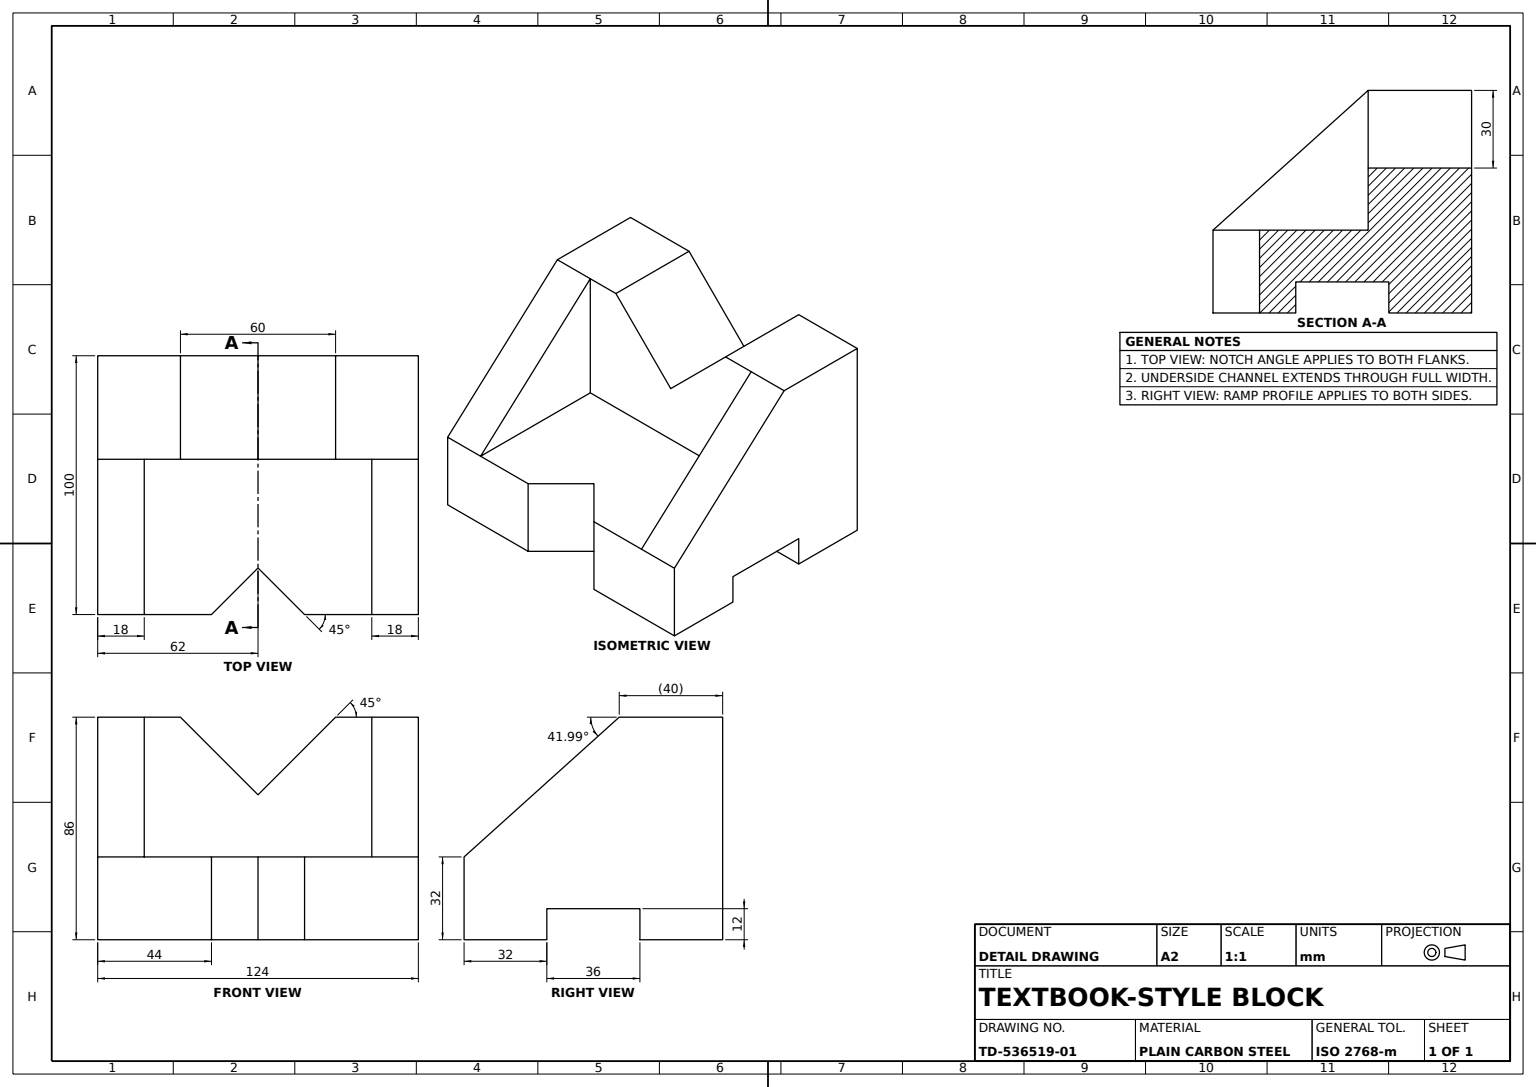
from build123d import *

# Parameters (mm, degrees)
V_BLOCK_BODY_100_DEPTH    = 100
CENTRAL_CHANNEL_SKETCH_W  = 36
CENTRAL_CHANNEL_SKETCH_H  = 12
CENTRAL_CHANNEL_CUT_DEPTH = 166
SQUARE_POCKET_18X18_REACH = 179.739
SQUARE_START              = -32
SQUARE_POCKET_SKETCH_W    = 88
SQUARE_POCKET_SKETCH_H    = 60
ANGLED_NOTCH_CUT_REACH    = 131.46


with BuildPart() as part:
    # V-Block Profile Sketch → V-Block Body 100 (new body)
    with BuildSketch(Plane.XY):
        Polygon((-30, 43), (0, 13), (30, 43), (62, 43), (62, -43), (-62, -43), (-62, 43), align=None)
    extrude(amount=V_BLOCK_BODY_100_DEPTH)

    # Central Channel Sketch → Central Channel Cut (cut, through all)
    with BuildSketch(Plane.ZY.offset(62)):
        with Locations((50, -37)):
            Rectangle(CENTRAL_CHANNEL_SKETCH_W, CENTRAL_CHANNEL_SKETCH_H)
        Polygon((40, 43), (100, -11), (100, 43), align=None)
    extrude(amount=-CENTRAL_CHANNEL_CUT_DEPTH, mode=Mode.SUBTRACT)

    # Square Pocket 18x18: up to this face of the body (flat: up to its plane)
    square_pocket_18x18_end = Plane(part.part.faces().sort_by_distance((-46, 43, 20))[0])
    # Square Pocket Sketch → Square Pocket 18x18 (cut, up to the picked face)
    with BuildSketch(Plane.XZ.offset(43).offset(SQUARE_START), mode=Mode.PRIVATE) as square_pocket_18x18_sk1:
        with Locations((0, 70)):
            Rectangle(SQUARE_POCKET_SKETCH_W, SQUARE_POCKET_SKETCH_H)
    square_pocket_18x18_tool1 = split(extrude(square_pocket_18x18_sk1.sketch, amount=-SQUARE_POCKET_18X18_REACH, mode=Mode.PRIVATE), bisect_by=square_pocket_18x18_end, keep=Keep.BOTH, mode=Mode.PRIVATE)
    add(square_pocket_18x18_tool1.solids().sort_by(Axis((0, -11, 70), (0, 1, 0)))[0], mode=Mode.SUBTRACT)

    # Angled Notch Sketch → Angled Notch Cut (cut, up to next)
    with BuildSketch(Plane(origin=(0, -11, 0), x_dir=(1, 0, 0), z_dir=(0, 1, 0)), mode=Mode.PRIVATE) as angled_notch_cut_sk1:
        Polygon((-18, -100), (0, -82), (18, -100), align=None)
    angled_notch_cut_tool1 = extrude(angled_notch_cut_sk1.sketch, amount=-ANGLED_NOTCH_CUT_REACH, mode=Mode.PRIVATE) & part.part
    add(angled_notch_cut_tool1.solids().sort_by_distance((0, -11, 94))[0], mode=Mode.SUBTRACT)


solid = part.part
